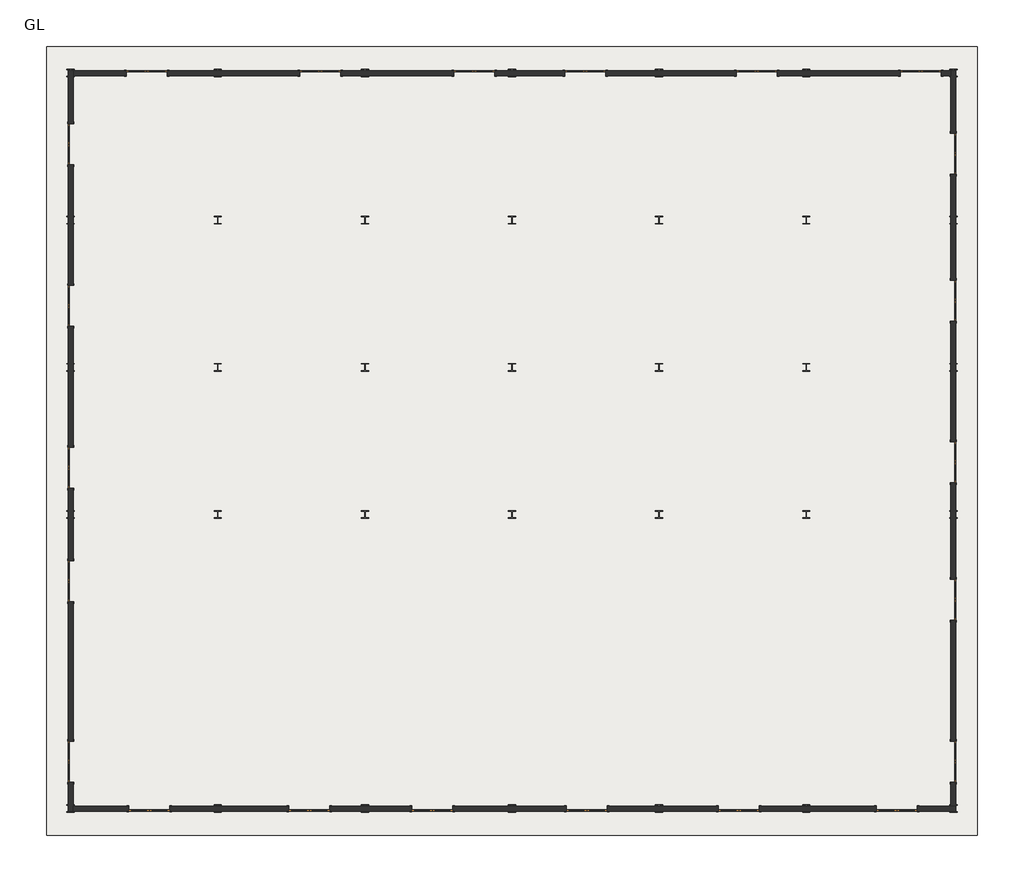
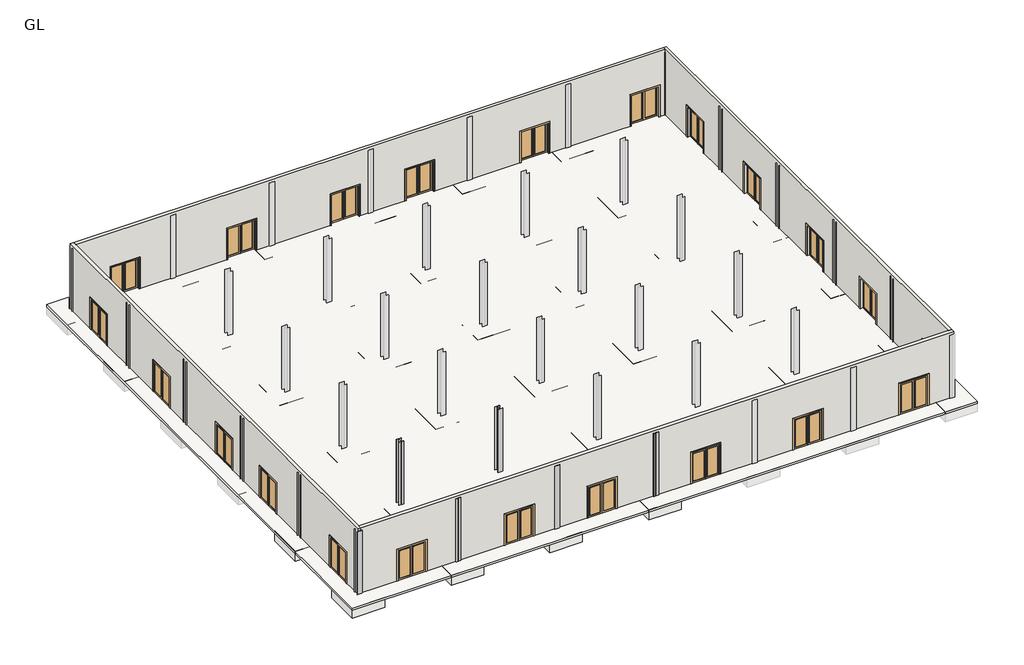
# One storey, part 1 of 2: 22 doors, 9 slabs, 7 columns, 4 walls.
"""IFC4 building model written with IfcOpenShell, lengths in millimetres."""

from ifc_helpers import new_model, si_unit, frame, origin, place, context, project, spatial, polyline, outline, extrude, faceted_brep, transform, mapped, element, save
from components import uc_universal_columns_column_uc305x305x97_28816581, m_door_double_glass_1700_x_2000mm_d5355b94, m_footing_rectangular_2200_x_2000_x_650mm_2_4a7b59ae

model = new_model("IFC4")

# Units and contexts
model_context = context("Model", 3, world=origin())
ifc_project = project(units=[si_unit("LENGTHUNIT", "METRE", prefix="MILLI")], contexts=[model_context])

# Site, building, storey
site = spatial("IfcSite", under=ifc_project)
building = spatial("IfcBuilding", under=site)
storey = spatial("IfcBuildingStorey", under=building, Name="GL", Elevation=-1812.3304639)

# Columns
placement = place(None, origin())
uc_universal_columns_column_uc305x305x97_shape = uc_universal_columns_column_uc305x305x97_28816581(model_context)
element("IfcColumn", 1, ObjectType="UC-Universal Columns-Column : UC305x305x97", at=placement, inside=storey, context=model_context, shape_type="MappedRepresentation", body=[
    mapped(uc_universal_columns_column_uc305x305x97_shape, transform((-18630.5493858, -6191.7308265, 0.0), x_axis=(1.0, 0.0, 0.0), y_axis=(0.0, 1.0, 0.0), z_axis=(0.0, 0.0, 1.0))),
])
element("IfcColumn", 2, ObjectType="UC-Universal Columns-Column : UC305x305x97", at=placement, inside=storey, context=model_context, shape_type="MappedRepresentation", body=[
    mapped(uc_universal_columns_column_uc305x305x97_shape, transform((-12534.5493858, -6191.7308265, 0.0), x_axis=(1.0, 0.0, 0.0), y_axis=(0.0, 1.0, 0.0), z_axis=(0.0, 0.0, 1.0))),
])
element("IfcColumn", 3, ObjectType="UC-Universal Columns-Column : UC305x305x97", at=placement, inside=storey, context=model_context, shape_type="MappedRepresentation", body=[
    mapped(uc_universal_columns_column_uc305x305x97_shape, transform((-6438.5493858, -6191.7308265, 0.0), x_axis=(1.0, 0.0, 0.0), y_axis=(0.0, 1.0, 0.0), z_axis=(0.0, 0.0, 1.0))),
])
element("IfcColumn", 4, ObjectType="UC-Universal Columns-Column : UC305x305x97", at=placement, inside=storey, context=model_context, shape_type="MappedRepresentation", body=[
    mapped(uc_universal_columns_column_uc305x305x97_shape, transform((-342.5493858, -6191.7308265, 0.0), x_axis=(1.0, 0.0, 0.0), y_axis=(0.0, 1.0, 0.0), z_axis=(0.0, 0.0, 1.0))),
])
element("IfcColumn", 5, ObjectType="UC-Universal Columns-Column : UC305x305x97", at=placement, inside=storey, context=model_context, shape_type="MappedRepresentation", body=[
    mapped(uc_universal_columns_column_uc305x305x97_shape, transform((-18630.5493858, -95.7308265, 0.0), x_axis=(1.0, 0.0, 0.0), y_axis=(0.0, 1.0, 0.0), z_axis=(0.0, 0.0, 1.0))),
])
element("IfcColumn", 6, ObjectType="UC-Universal Columns-Column : UC305x305x97", at=placement, inside=storey, context=model_context, shape_type="MappedRepresentation", body=[
    mapped(uc_universal_columns_column_uc305x305x97_shape, transform((-12534.5493858, -95.7308265, 0.0), x_axis=(1.0, 0.0, 0.0), y_axis=(0.0, 1.0, 0.0), z_axis=(0.0, 0.0, 1.0))),
])
element("IfcColumn", 7, ObjectType="UC-Universal Columns-Column : UC305x305x97", at=placement, inside=storey, context=model_context, shape_type="MappedRepresentation", body=[
    mapped(uc_universal_columns_column_uc305x305x97_shape, transform((-6438.5493858, -95.7308265, 0.0), x_axis=(1.0, 0.0, 0.0), y_axis=(0.0, 1.0, 0.0), z_axis=(0.0, 0.0, 1.0))),
])

# Doors
m_door_double_glass_1700_x_2000mm_shape = m_door_double_glass_1700_x_2000mm_d5355b94(model_context)
element("IfcDoor", 8, ObjectType="M_Door-Double-Glass : 1700 x 2000mm", at=placement, inside=storey, context=model_context, shape_type="MappedRepresentation", body=[
    mapped(m_door_double_glass_1700_x_2000mm_shape, transform((-3650.2445858, -6189.3495765, -1812.3304639), x_axis=(-1.0, 0.0, 0.0), y_axis=(0.0, -1.0, 0.0), z_axis=(0.0, 0.0, 1.0))),
])
element("IfcDoor", 9, ObjectType="M_Door-Double-Glass : 1700 x 2000mm", at=placement, inside=storey, context=model_context, shape_type="MappedRepresentation", body=[
    mapped(m_door_double_glass_1700_x_2000mm_shape, transform((2749.7554142, -6189.3495765, -1812.3304639), x_axis=(-1.0, 0.0, 0.0), y_axis=(0.0, -1.0, 0.0), z_axis=(0.0, 0.0, 1.0))),
])
element("IfcDoor", 10, ObjectType="M_Door-Double-Glass : 1700 x 2000mm", at=placement, inside=storey, context=model_context, shape_type="MappedRepresentation", body=[
    mapped(m_door_double_glass_1700_x_2000mm_shape, transform((-8292.3969858, 24285.5831235, -1812.3304639), x_axis=(1.0, 0.0, 0.0), y_axis=(0.0, 1.0, 0.0), z_axis=(0.0, 0.0, 1.0))),
])
element("IfcDoor", 11, ObjectType="M_Door-Double-Glass : 1700 x 2000mm", at=placement, inside=storey, context=model_context, shape_type="MappedRepresentation", body=[
    mapped(m_door_double_glass_1700_x_2000mm_shape, transform((9795.4506142, 24285.5831235, -1812.3304639), x_axis=(1.0, 0.0, 0.0), y_axis=(0.0, 1.0, 0.0), z_axis=(0.0, 0.0, 1.0))),
])
element("IfcDoor", 12, ObjectType="M_Door-Double-Glass : 1700 x 2000mm", at=placement, inside=storey, context=model_context, shape_type="MappedRepresentation", body=[
    mapped(m_door_double_glass_1700_x_2000mm_shape, transform((-15480.2445858, 24285.5831235, -1812.3304639), x_axis=(1.0, 0.0, 0.0), y_axis=(0.0, 1.0, 0.0), z_axis=(0.0, 0.0, 1.0))),
])
element("IfcDoor", 13, ObjectType="M_Door-Double-Glass : 1700 x 2000mm", at=placement, inside=storey, context=model_context, shape_type="MappedRepresentation", body=[
    mapped(m_door_double_glass_1700_x_2000mm_shape, transform((-1904.5493858, 24285.5831235, -1812.3304639), x_axis=(1.0, 0.0, 0.0), y_axis=(0.0, 1.0, 0.0), z_axis=(0.0, 0.0, 1.0))),
])
element("IfcDoor", 14, ObjectType="M_Door-Double-Glass : 1700 x 2000mm", at=placement, inside=storey, context=model_context, shape_type="MappedRepresentation", body=[
    mapped(m_door_double_glass_1700_x_2000mm_shape, transform((16595.4506142, 24285.5831235, -1812.3304639), x_axis=(1.0, 0.0, 0.0), y_axis=(0.0, 1.0, 0.0), z_axis=(0.0, 0.0, 1.0))),
])
element("IfcDoor", 15, ObjectType="M_Door-Double-Glass : 1700 x 2000mm", at=placement, inside=storey, context=model_context, shape_type="MappedRepresentation", body=[
    mapped(m_door_double_glass_1700_x_2000mm_shape, transform((2695.4506142, 24285.5831235, -1812.3304639), x_axis=(1.0, 0.0, 0.0), y_axis=(0.0, 1.0, 0.0), z_axis=(0.0, 0.0, 1.0))),
])
element("IfcDoor", 16, ObjectType="M_Door-Double-Glass : 1700 x 2000mm", at=placement, inside=storey, context=model_context, shape_type="MappedRepresentation", body=[
    mapped(m_door_double_glass_1700_x_2000mm_shape, transform((-18627.8633358, 21337.9643735, -1812.3304639), x_axis=(0.0, 1.0, 0.0), y_axis=(-1.0, 0.0, 0.0), z_axis=(0.0, 0.0, 1.0))),
])
element("IfcDoor", 17, ObjectType="M_Door-Double-Glass : 1700 x 2000mm", at=placement, inside=storey, context=model_context, shape_type="MappedRepresentation", body=[
    mapped(m_door_double_glass_1700_x_2000mm_shape, transform((-18627.8633358, 14637.9643735, -1812.3304639), x_axis=(0.0, 1.0, 0.0), y_axis=(-1.0, 0.0, 0.0), z_axis=(0.0, 0.0, 1.0))),
])
element("IfcDoor", 18, ObjectType="M_Door-Double-Glass : 1700 x 2000mm", at=placement, inside=storey, context=model_context, shape_type="MappedRepresentation", body=[
    mapped(m_door_double_glass_1700_x_2000mm_shape, transform((-18627.8633358, 7937.9643735, -1812.3304639), x_axis=(0.0, 1.0, 0.0), y_axis=(-1.0, 0.0, 0.0), z_axis=(0.0, 0.0, 1.0))),
])
element("IfcDoor", 19, ObjectType="M_Door-Double-Glass : 1700 x 2000mm", at=placement, inside=storey, context=model_context, shape_type="MappedRepresentation", body=[
    mapped(m_door_double_glass_1700_x_2000mm_shape, transform((-18627.8633358, 3237.9643735, -1812.3304639), x_axis=(0.0, 1.0, 0.0), y_axis=(-1.0, 0.0, 0.0), z_axis=(0.0, 0.0, 1.0))),
])
element("IfcDoor", 20, ObjectType="M_Door-Double-Glass : 1700 x 2000mm", at=placement, inside=storey, context=model_context, shape_type="MappedRepresentation", body=[
    mapped(m_door_double_glass_1700_x_2000mm_shape, transform((-18627.8633358, -4241.7308265, -1812.3304639), x_axis=(0.0, 1.0, 0.0), y_axis=(-1.0, 0.0, 0.0), z_axis=(0.0, 0.0, 1.0))),
])
element("IfcDoor", 21, ObjectType="M_Door-Double-Glass : 1700 x 2000mm", at=placement, inside=storey, context=model_context, shape_type="MappedRepresentation", body=[
    mapped(m_door_double_glass_1700_x_2000mm_shape, transform((17943.0693642, -4241.7308265, -1812.3304639), x_axis=(0.0, -1.0, 0.0), y_axis=(1.0, 0.0, 0.0), z_axis=(0.0, 0.0, 1.0))),
])
element("IfcDoor", 22, ObjectType="M_Door-Double-Glass : 1700 x 2000mm", at=placement, inside=storey, context=model_context, shape_type="MappedRepresentation", body=[
    mapped(m_door_double_glass_1700_x_2000mm_shape, transform((17943.0693642, 2458.2691735, -1812.3304639), x_axis=(0.0, -1.0, 0.0), y_axis=(1.0, 0.0, 0.0), z_axis=(0.0, 0.0, 1.0))),
])
element("IfcDoor", 23, ObjectType="M_Door-Double-Glass : 1700 x 2000mm", at=placement, inside=storey, context=model_context, shape_type="MappedRepresentation", body=[
    mapped(m_door_double_glass_1700_x_2000mm_shape, transform((17943.0693642, 8158.2691735, -1812.3304639), x_axis=(0.0, -1.0, 0.0), y_axis=(1.0, 0.0, 0.0), z_axis=(0.0, 0.0, 1.0))),
])
element("IfcDoor", 24, ObjectType="M_Door-Double-Glass : 1700 x 2000mm", at=placement, inside=storey, context=model_context, shape_type="MappedRepresentation", body=[
    mapped(m_door_double_glass_1700_x_2000mm_shape, transform((17943.0693642, 14858.2691735, -1812.3304639), x_axis=(0.0, -1.0, 0.0), y_axis=(1.0, 0.0, 0.0), z_axis=(0.0, 0.0, 1.0))),
])
element("IfcDoor", 25, ObjectType="M_Door-Double-Glass : 1700 x 2000mm", at=placement, inside=storey, context=model_context, shape_type="MappedRepresentation", body=[
    mapped(m_door_double_glass_1700_x_2000mm_shape, transform((-15380.2445858, -6189.3495765, -1812.3304639), x_axis=(-1.0, 0.0, 0.0), y_axis=(0.0, -1.0, 0.0), z_axis=(0.0, 0.0, 1.0))),
])
element("IfcDoor", 26, ObjectType="M_Door-Double-Glass : 1700 x 2000mm", at=placement, inside=storey, context=model_context, shape_type="MappedRepresentation", body=[
    mapped(m_door_double_glass_1700_x_2000mm_shape, transform((-8750.2445858, -6189.3495765, -1812.3304639), x_axis=(-1.0, 0.0, 0.0), y_axis=(0.0, -1.0, 0.0), z_axis=(0.0, 0.0, 1.0))),
])
element("IfcDoor", 27, ObjectType="M_Door-Double-Glass : 1700 x 2000mm", at=placement, inside=storey, context=model_context, shape_type="MappedRepresentation", body=[
    mapped(m_door_double_glass_1700_x_2000mm_shape, transform((9049.7554142, -6189.3495765, -1812.3304639), x_axis=(-1.0, 0.0, 0.0), y_axis=(0.0, -1.0, 0.0), z_axis=(0.0, 0.0, 1.0))),
])
element("IfcDoor", 28, ObjectType="M_Door-Double-Glass : 1700 x 2000mm", at=placement, inside=storey, context=model_context, shape_type="MappedRepresentation", body=[
    mapped(m_door_double_glass_1700_x_2000mm_shape, transform((15595.4506142, -6189.3495765, -1812.3304639), x_axis=(-1.0, 0.0, 0.0), y_axis=(0.0, -1.0, 0.0), z_axis=(0.0, 0.0, 1.0))),
])
element("IfcDoor", 29, ObjectType="M_Door-Double-Glass : 1700 x 2000mm", at=placement, inside=storey, context=model_context, shape_type="MappedRepresentation", body=[
    mapped(m_door_double_glass_1700_x_2000mm_shape, transform((17943.0693642, 20937.9643735, -1812.3304639), x_axis=(0.0, -1.0, 0.0), y_axis=(1.0, 0.0, 0.0), z_axis=(0.0, 0.0, 1.0))),
])

# Slabs
element("IfcSlab", 30, ObjectType="Generic 150mm", at=placement, inside=storey, context=model_context, shape_type="SweptSolid", body=[
    extrude(outline(polyline([(18945.4506142, 25388.2691735), (18945.4506142, -7291.7308265), (-19630.5493858, -7291.7308265), (-19630.5493858, 25388.2691735), (18945.4506142, 25388.2691735)])), frame((0.0, 0.0, -1962.3304639), z_axis=(0.0, 0.0, 1.0), x_axis=(1.0, 0.0, 0.0)), (0.0, 0.0, 1.0), 150.0),
])
m_footing_rectangular_2200_x_2000_x_650mm_2_shape = m_footing_rectangular_2200_x_2000_x_650mm_2_4a7b59ae(model_context)
element("IfcSlab", 31, ObjectType="M_Footing-Rectangular : 2200 x 2000 x 650mm 2", at=placement, inside=storey, context=model_context, shape_type="MappedRepresentation", body=[
    mapped(m_footing_rectangular_2200_x_2000_x_650mm_2_shape, transform((-18630.5493858, -6191.7308265, -1812.3304639), x_axis=(1.0, 0.0, 0.0), y_axis=(0.0, 1.0, 0.0), z_axis=(0.0, 0.0, 1.0))),
])
element("IfcSlab", 32, ObjectType="M_Footing-Rectangular : 2200 x 2000 x 650mm 2", at=placement, inside=storey, context=model_context, shape_type="MappedRepresentation", body=[
    mapped(m_footing_rectangular_2200_x_2000_x_650mm_2_shape, transform((-12534.5493858, -6191.7308265, -1812.3304639), x_axis=(1.0, 0.0, 0.0), y_axis=(0.0, 1.0, 0.0), z_axis=(0.0, 0.0, 1.0))),
])
element("IfcSlab", 33, ObjectType="M_Footing-Rectangular : 2200 x 2000 x 650mm 2", at=placement, inside=storey, context=model_context, shape_type="MappedRepresentation", body=[
    mapped(m_footing_rectangular_2200_x_2000_x_650mm_2_shape, transform((-6438.5493858, -6191.7308265, -1812.3304639), x_axis=(1.0, 0.0, 0.0), y_axis=(0.0, 1.0, 0.0), z_axis=(0.0, 0.0, 1.0))),
])
element("IfcSlab", 34, ObjectType="M_Footing-Rectangular : 2200 x 2000 x 650mm 2", at=placement, inside=storey, context=model_context, shape_type="MappedRepresentation", body=[
    mapped(m_footing_rectangular_2200_x_2000_x_650mm_2_shape, transform((-342.5493858, -6191.7308265, -1812.3304639), x_axis=(1.0, 0.0, 0.0), y_axis=(0.0, 1.0, 0.0), z_axis=(0.0, 0.0, 1.0))),
])
element("IfcSlab", 35, ObjectType="M_Footing-Rectangular : 2200 x 2000 x 650mm 2", at=placement, inside=storey, context=model_context, shape_type="MappedRepresentation", body=[
    mapped(m_footing_rectangular_2200_x_2000_x_650mm_2_shape, transform((-18630.5493858, -95.7308265, -1812.3304639), x_axis=(1.0, 0.0, 0.0), y_axis=(0.0, 1.0, 0.0), z_axis=(0.0, 0.0, 1.0))),
])
element("IfcSlab", 36, ObjectType="M_Footing-Rectangular : 2200 x 2000 x 650mm 2", at=placement, inside=storey, context=model_context, shape_type="MappedRepresentation", body=[
    mapped(m_footing_rectangular_2200_x_2000_x_650mm_2_shape, transform((-12534.5493858, -95.7308265, -1812.3304639), x_axis=(1.0, 0.0, 0.0), y_axis=(0.0, 1.0, 0.0), z_axis=(0.0, 0.0, 1.0))),
])
element("IfcSlab", 37, ObjectType="M_Footing-Rectangular : 2200 x 2000 x 650mm 2", at=placement, inside=storey, context=model_context, shape_type="MappedRepresentation", body=[
    mapped(m_footing_rectangular_2200_x_2000_x_650mm_2_shape, transform((-6438.5493858, -95.7308265, -1812.3304639), x_axis=(1.0, 0.0, 0.0), y_axis=(0.0, 1.0, 0.0), z_axis=(0.0, 0.0, 1.0))),
])
element("IfcSlab", 38, ObjectType="M_Footing-Rectangular : 2200 x 2000 x 650mm 2", at=placement, inside=storey, context=model_context, shape_type="MappedRepresentation", body=[
    mapped(m_footing_rectangular_2200_x_2000_x_650mm_2_shape, transform((-342.5493858, -95.7308265, -1812.3304639), x_axis=(1.0, 0.0, 0.0), y_axis=(0.0, 1.0, 0.0), z_axis=(0.0, 0.0, 1.0))),
])

# Walls
element("IfcWall", 39, ObjectType="Generic - 200mm", at=placement, inside=storey, context=model_context, shape_type="Brep", body=[
    faceted_brep([(-18730.2445858, 2387.9643735, -1812.3304639), (-18730.2445858, -3391.7308265, -1812.3304639), (-18730.2445858, -3391.7308265, 187.6695361), (-18730.2445858, -5091.7308265, 187.6695361), (-18730.2445858, -5091.7308265, -1812.3304639), (-18730.2445858, -6291.7308265, -1812.3304639), (-18730.2445858, -6291.7308265, 2454.6695361), (-18730.2445858, 24387.9643735, 2454.6695361), (-18730.2445858, 24387.9643735, -1812.3304639), (-18730.2445858, 22187.9643735, -1812.3304639), (-18730.2445858, 22187.9643735, 187.6695361), (-18730.2445858, 20487.9643735, 187.6695361), (-18730.2445858, 20487.9643735, -1812.3304639), (-18730.2445858, 15487.9643735, -1812.3304639), (-18730.2445858, 15487.9643735, 187.6695361), (-18730.2445858, 13787.9643735, 187.6695361), (-18730.2445858, 13787.9643735, -1812.3304639), (-18730.2445858, 8787.9643735, -1812.3304639), (-18730.2445858, 8787.9643735, 187.6695361), (-18730.2445858, 7087.9643735, 187.6695361), (-18730.2445858, 7087.9643735, -1812.3304639), (-18730.2445858, 4087.9643735, -1812.3304639), (-18730.2445858, 4087.9643735, 187.6695361), (-18730.2445858, 2387.9643735, 187.6695361), (-18530.2445858, -3391.7308265, 187.6695361), (-18530.2445858, -3391.7308265, -1812.3304639), (-18530.2445858, 2387.9643735, -1812.3304639), (-18530.2445858, 2387.9643735, 187.6695361), (-18530.2445858, 4087.9643735, 187.6695361), (-18530.2445858, 4087.9643735, -1812.3304639), (-18530.2445858, 7087.9643735, -1812.3304639), (-18530.2445858, 7087.9643735, 187.6695361), (-18530.2445858, 8787.9643735, 187.6695361), (-18530.2445858, 8787.9643735, -1812.3304639), (-18530.2445858, 13787.9643735, -1812.3304639), (-18530.2445858, 13787.9643735, 187.6695361), (-18530.2445858, 15487.9643735, 187.6695361), (-18530.2445858, 15487.9643735, -1812.3304639), (-18530.2445858, 20487.9643735, -1812.3304639), (-18530.2445858, 20487.9643735, 187.6695361), (-18530.2445858, 22187.9643735, 187.6695361), (-18530.2445858, 22187.9643735, -1812.3304639), (-18530.2445858, 24187.9643735, -1812.3304639), (-18530.2445858, 24387.9643735, -1812.3304639), (-18530.2445858, 24387.9643735, 2454.6695361), (-18530.2445858, 24187.9643735, 2454.6695361), (-18530.2445858, -6091.7308265, 2454.6695361), (-18530.2445858, -6291.7308265, 2454.6695361), (-18530.2445858, -6291.7308265, -1812.3304639), (-18530.2445858, -6091.7308265, -1812.3304639), (-18530.2445858, -5091.7308265, -1812.3304639), (-18530.2445858, -5091.7308265, 187.6695361)], [[[0, 1, 2, 3, 4, 5, 6, 7, 8, 9, 10, 11, 12, 13, 14, 15, 16, 17, 18, 19, 20, 21, 22, 23]], [[24, 25, 26, 27, 28, 29, 30, 31, 32, 33, 34, 35, 36, 37, 38, 39, 40, 41, 42, 43, 44, 45, 46, 47, 48, 49, 50, 51]], [[43, 42, 41, 9, 8]], [[38, 37, 13, 12]], [[34, 33, 17, 16]], [[30, 29, 21, 20]], [[26, 25, 1, 0]], [[50, 49, 48, 5, 4]], [[7, 6, 47, 46, 45, 44]], [[6, 5, 48, 47]], [[8, 7, 44, 43]], [[10, 9, 41, 40]], [[11, 10, 40, 39]], [[12, 11, 39, 38]], [[14, 13, 37, 36]], [[15, 14, 36, 35]], [[16, 15, 35, 34]], [[18, 17, 33, 32]], [[19, 18, 32, 31]], [[20, 19, 31, 30]], [[22, 21, 29, 28]], [[23, 22, 28, 27]], [[0, 23, 27, 26]], [[2, 1, 25, 24]], [[3, 2, 24, 51]], [[4, 3, 51, 50]]]),
])
element("IfcWall", 40, ObjectType="Generic - 200mm", at=placement, inside=storey, context=model_context, shape_type="Brep", body=[
    faceted_brep([(9899.7554142, -6291.7308265, -1812.3304639), (14745.4506142, -6291.7308265, -1812.3304639), (14745.4506142, -6291.7308265, 187.6695361), (16445.4506142, -6291.7308265, 187.6695361), (16445.4506142, -6291.7308265, -1812.3304639), (18045.4506142, -6291.7308265, -1812.3304639), (18045.4506142, -6291.7308265, 2454.6695361), (-18530.2445858, -6291.7308265, 2454.6695361), (-18530.2445858, -6291.7308265, -1812.3304639), (-16230.2445858, -6291.7308265, -1812.3304639), (-16230.2445858, -6291.7308265, 187.6695361), (-14530.2445858, -6291.7308265, 187.6695361), (-14530.2445858, -6291.7308265, -1812.3304639), (-9600.2445858, -6291.7308265, -1812.3304639), (-9600.2445858, -6291.7308265, 187.6695361), (-7900.2445858, -6291.7308265, 187.6695361), (-7900.2445858, -6291.7308265, -1812.3304639), (-4500.2445858, -6291.7308265, -1812.3304639), (-4500.2445858, -6291.7308265, 187.6695361), (-2800.2445858, -6291.7308265, 187.6695361), (-2800.2445858, -6291.7308265, -1812.3304639), (1899.7554142, -6291.7308265, -1812.3304639), (1899.7554142, -6291.7308265, 187.6695361), (3599.7554142, -6291.7308265, 187.6695361), (3599.7554142, -6291.7308265, -1812.3304639), (8199.7554142, -6291.7308265, -1812.3304639), (8199.7554142, -6291.7308265, 187.6695361), (9899.7554142, -6291.7308265, 187.6695361), (14745.4506142, -6091.7308265, 187.6695361), (14745.4506142, -6091.7308265, -1812.3304639), (9899.7554142, -6091.7308265, -1812.3304639), (9899.7554142, -6091.7308265, 187.6695361), (8199.7554142, -6091.7308265, 187.6695361), (8199.7554142, -6091.7308265, -1812.3304639), (3599.7554142, -6091.7308265, -1812.3304639), (3599.7554142, -6091.7308265, 187.6695361), (1899.7554142, -6091.7308265, 187.6695361), (1899.7554142, -6091.7308265, -1812.3304639), (-2800.2445858, -6091.7308265, -1812.3304639), (-2800.2445858, -6091.7308265, 187.6695361), (-4500.2445858, -6091.7308265, 187.6695361), (-4500.2445858, -6091.7308265, -1812.3304639), (-7900.2445858, -6091.7308265, -1812.3304639), (-7900.2445858, -6091.7308265, 187.6695361), (-9600.2445858, -6091.7308265, 187.6695361), (-9600.2445858, -6091.7308265, -1812.3304639), (-14530.2445858, -6091.7308265, -1812.3304639), (-14530.2445858, -6091.7308265, 187.6695361), (-16230.2445858, -6091.7308265, 187.6695361), (-16230.2445858, -6091.7308265, -1812.3304639), (-18530.2445858, -6091.7308265, -1812.3304639), (-18530.2445858, -6091.7308265, 2454.6695361), (17845.4506142, -6091.7308265, 2454.6695361), (18045.4506142, -6091.7308265, 2454.6695361), (18045.4506142, -6091.7308265, -1812.3304639), (17845.4506142, -6091.7308265, -1812.3304639), (16445.4506142, -6091.7308265, -1812.3304639), (16445.4506142, -6091.7308265, 187.6695361)], [[[0, 1, 2, 3, 4, 5, 6, 7, 8, 9, 10, 11, 12, 13, 14, 15, 16, 17, 18, 19, 20, 21, 22, 23, 24, 25, 26, 27]], [[28, 29, 30, 31, 32, 33, 34, 35, 36, 37, 38, 39, 40, 41, 42, 43, 44, 45, 46, 47, 48, 49, 50, 51, 52, 53, 54, 55, 56, 57]], [[38, 37, 21, 20]], [[50, 49, 9, 8]], [[42, 41, 17, 16]], [[46, 45, 13, 12]], [[34, 33, 25, 24]], [[30, 29, 1, 0]], [[56, 55, 54, 5, 4]], [[7, 6, 53, 52, 51]], [[8, 7, 51, 50]], [[6, 5, 54, 53]], [[18, 17, 41, 40]], [[19, 18, 40, 39]], [[20, 19, 39, 38]], [[22, 21, 37, 36]], [[23, 22, 36, 35]], [[24, 23, 35, 34]], [[10, 9, 49, 48]], [[11, 10, 48, 47]], [[12, 11, 47, 46]], [[14, 13, 45, 44]], [[15, 14, 44, 43]], [[16, 15, 43, 42]], [[26, 25, 33, 32]], [[27, 26, 32, 31]], [[0, 27, 31, 30]], [[2, 1, 29, 28]], [[3, 2, 28, 57]], [[4, 3, 57, 56]]]),
])
element("IfcWall", 41, ObjectType="Generic - 200mm", at=placement, inside=storey, context=model_context, shape_type="Brep", body=[
    faceted_brep([(18045.4506142, 15708.2691735, -1812.3304639), (18045.4506142, 20087.9643735, -1812.3304639), (18045.4506142, 20087.9643735, 187.6695361), (18045.4506142, 21787.9643735, 187.6695361), (18045.4506142, 21787.9643735, -1812.3304639), (18045.4506142, 24387.9643735, -1812.3304639), (18045.4506142, 24387.9643735, 2454.6695361), (18045.4506142, -6091.7308265, 2454.6695361), (18045.4506142, -6091.7308265, -1812.3304639), (18045.4506142, -5091.7308265, -1812.3304639), (18045.4506142, -5091.7308265, 187.6695361), (18045.4506142, -3391.7308265, 187.6695361), (18045.4506142, -3391.7308265, -1812.3304639), (18045.4506142, 1608.2691735, -1812.3304639), (18045.4506142, 1608.2691735, 187.6695361), (18045.4506142, 3308.2691735, 187.6695361), (18045.4506142, 3308.2691735, -1812.3304639), (18045.4506142, 7308.2691735, -1812.3304639), (18045.4506142, 7308.2691735, 187.6695361), (18045.4506142, 9008.2691735, 187.6695361), (18045.4506142, 9008.2691735, -1812.3304639), (18045.4506142, 14008.2691735, -1812.3304639), (18045.4506142, 14008.2691735, 187.6695361), (18045.4506142, 15708.2691735, 187.6695361), (17845.4506142, 20087.9643735, 187.6695361), (17845.4506142, 20087.9643735, -1812.3304639), (17845.4506142, 15708.2691735, -1812.3304639), (17845.4506142, 15708.2691735, 187.6695361), (17845.4506142, 14008.2691735, 187.6695361), (17845.4506142, 14008.2691735, -1812.3304639), (17845.4506142, 9008.2691735, -1812.3304639), (17845.4506142, 9008.2691735, 187.6695361), (17845.4506142, 7308.2691735, 187.6695361), (17845.4506142, 7308.2691735, -1812.3304639), (17845.4506142, 3308.2691735, -1812.3304639), (17845.4506142, 3308.2691735, 187.6695361), (17845.4506142, 1608.2691735, 187.6695361), (17845.4506142, 1608.2691735, -1812.3304639), (17845.4506142, -3391.7308265, -1812.3304639), (17845.4506142, -3391.7308265, 187.6695361), (17845.4506142, -5091.7308265, 187.6695361), (17845.4506142, -5091.7308265, -1812.3304639), (17845.4506142, -6091.7308265, -1812.3304639), (17845.4506142, -6091.7308265, 2454.6695361), (17845.4506142, 24187.9643735, 2454.6695361), (17845.4506142, 24387.9643735, 2454.6695361), (17845.4506142, 24387.9643735, -1812.3304639), (17845.4506142, 24187.9643735, -1812.3304639), (17845.4506142, 21787.9643735, -1812.3304639), (17845.4506142, 21787.9643735, 187.6695361)], [[[0, 1, 2, 3, 4, 5, 6, 7, 8, 9, 10, 11, 12, 13, 14, 15, 16, 17, 18, 19, 20, 21, 22, 23]], [[24, 25, 26, 27, 28, 29, 30, 31, 32, 33, 34, 35, 36, 37, 38, 39, 40, 41, 42, 43, 44, 45, 46, 47, 48, 49]], [[42, 41, 9, 8]], [[38, 37, 13, 12]], [[34, 33, 17, 16]], [[30, 29, 21, 20]], [[26, 25, 1, 0]], [[48, 47, 46, 5, 4]], [[7, 6, 45, 44, 43]], [[8, 7, 43, 42]], [[6, 5, 46, 45]], [[10, 9, 41, 40]], [[11, 10, 40, 39]], [[12, 11, 39, 38]], [[14, 13, 37, 36]], [[15, 14, 36, 35]], [[16, 15, 35, 34]], [[18, 17, 33, 32]], [[19, 18, 32, 31]], [[20, 19, 31, 30]], [[22, 21, 29, 28]], [[23, 22, 28, 27]], [[0, 23, 27, 26]], [[2, 1, 25, 24]], [[3, 2, 24, 49]], [[4, 3, 49, 48]]]),
])
element("IfcWall", 42, ObjectType="Generic - 200mm", at=placement, inside=storey, context=model_context, shape_type="SweptSolid", body=[
    extrude(outline(polyline([(187.6695361, 3545.4506142), (-1812.3304639, 3545.4506142), (-1812.3304639, 8945.4506142), (187.6695361, 8945.4506142), (187.6695361, 10645.4506142), (-1812.3304639, 10645.4506142), (-1812.3304639, 15745.4506142), (187.6695361, 15745.4506142), (187.6695361, 17445.4506142), (-1812.3304639, 17445.4506142), (-1812.3304639, 17845.4506142), (2454.6695361, 17845.4506142), (2454.6695361, -18530.2445858), (-1812.3304639, -18530.2445858), (-1812.3304639, -16330.2445858), (187.6695361, -16330.2445858), (187.6695361, -14630.2445858), (-1812.3304639, -14630.2445858), (-1812.3304639, -9142.3969858), (187.6695361, -9142.3969858), (187.6695361, -7442.3969858), (-1812.3304639, -7442.3969858), (-1812.3304639, -2754.5493858), (187.6695361, -2754.5493858), (187.6695361, -1054.5493858), (-1812.3304639, -1054.5493858), (-1812.3304639, 1845.4506142), (187.6695361, 1845.4506142), (187.6695361, 3545.4506142)])), frame((0.0, 24187.9643735, 0.0), z_axis=(0.0, 1.0, 0.0), x_axis=(0.0, 0.0, 1.0)), (0.0, 0.0, 1.0), 200.0),
])

save(model, "model.ifc")

# Revit data of these elements
# Grids (mm)
#   "1": line (20610.061, -6191.731) -> (-20257.131, -6191.731)
#   "2": line (20610.061, -95.731) -> (-20257.131, -95.731)
#   "3": line (20610.061, 6000.269) -> (-20257.131, 6000.269)
#   "4": line (20610.061, 12096.269) -> (-20257.131, 12096.269)
#   "5": line (20610.061, 18192.269) -> (-20257.131, 18192.269)
#   "6": line (20610.061, 24288.269) -> (-20257.131, 24288.269)
#   "8": line (-12534.549, 28626.482) -> (-12534.549, -10472.495)
#   "9": line (-6438.549, 28626.482) -> (-6438.549, -10472.495)
#   "10": line (-342.549, 28626.482) -> (-342.549, -10472.495)
#   "11": line (5753.451, 28626.482) -> (5753.451, -10472.495)
#   "12": line (11849.451, 28626.482) -> (11849.451, -10472.495)
#   "13": line (17945.451, 28626.482) -> (17945.451, -10472.495)
#   "7": line (-18630.549, 28626.482) -> (-18630.549, -10472.495)
# Type "UC-Universal Columns-Column : UC305x305x97"
#   Section Name Key = "UC305x305x97"
#   Width = 30.53 cm
#   Web Thickness = 0.99 cm
#   Web Fillet = 1.52 cm
#   Warping Constant = 1560000.0 cm⁶
#   Torsional Moment of Inertia = 91.20 cm⁴
#   Section Area = 123.0 cm²
#   Plastic Modulus weak axis = 726.0 cm³
#   Plastic Modulus strong axis = 1592.0 cm³
#   Nominal Weight = 96.8996 kgf/m
#   Moment of Inertia weak axis = 7308.00 cm⁴
#   Moment of Inertia strong axis = 22249.00 cm⁴
#   Height = 30.79 cm
#   Flange Thickness = 1.54 cm
#   Elastic Modulus weak axis = 479.0 cm³
#   Elastic Modulus strong axis = 1445.0 cm³
#   Centroid Vertical = 15.395 cm
#   Centroid Horizontal = 15.265 cm
#   Bolt Spacing = 14.0 cm
#   Structural Material [instance default] = Metal - Steel 43-275
#   Type Comments = ""
#   Assembly Code = ""
# Type "M_Door-Double-Glass : 1700 x 2000mm"
#   Type Mark = "40"
#   Construction Type Id = "opn-d45"
#   Assembly Code = "C1020"
#   Analytic Construction = "Wood frame, double glass door "
#   W = 850 mm
#   Thickness = 50 mm
#   Thermal Resistance (R) = 0.31964 (m²·K)/W
#   Swing Angle [instance default] = 90.00°
#   Heat Transfer Coefficient (U) = 3.12872 W/(m²·K)
#   Height = 2000 mm
#   Bottom Rail = 100 mm
#   Top Rail = 100 mm
#   Stiles = 100 mm
#   Trim Projection = 25 mm
#   Trim Width = 80 mm
#   Width = 1700 mm
#   Define Thermal Properties by = 1
#   Glazing = Glass
#   Panel Material = Wood - Birch - Solid Stained Light Low Gloss
#   Trim Material = Paint - Sienna
#   Visual Light Transmittance = 0
#   Solar Heat Gain Coefficient = 0
#   Function = (empty or 0)
#   Wall Closure = (empty or 0)
# Type "Generic 150mm"
#   Function = 0
#   Layers, outside or top first: 150 mm "Render, Tan, Textured" (function 1)
# Type "M_Footing-Rectangular : 2200 x 2000 x 650mm 2"
#   Width = 2000 mm
#   Length = 2200 mm
#   Foundation Thickness = 650 mm
#   Structural Material [instance default] = Concrete, Cast-in-Place gray
#   Assembly Code = ""
# Type "Generic - 200mm"
#   Layers, outside or top first: 200 mm "Door - Frame" (function 1)
# Elements 1, 2, 3, 4, 5, 6, 7 (IfcColumn, "UC-Universal Columns-Column : UC305x305x97")
#   Structural Material = Metal - Steel 43-275
#   Phase Created = New Construction
#   Materials on its faces: "Metal - Steel 43-275"
# Elements 8, 9, 10, 11, 12, 13, 14, 15, 16, 17, 18, 19, 20, 21, 22, 23, 24, 25, 26, 27, 28, 29 (IfcDoor, "M_Door-Double-Glass : 1700 x 2000mm")
#   Swing Angle = 90.00°
#   Phase Created = New Construction
#   Materials on its faces: "Wood - Birch - Solid Stained Light Low Gloss", "Paint - Sienna", "Glass"
# Element 30 (IfcSlab, "Generic 150mm")
#   Height Offset From Level = 0 mm
#   Phase Created = New Construction
#   Materials on its faces: "Render, Tan, Textured"
# Elements 31, 32, 33, 34, 35, 36, 37, 38 (IfcSlab, "M_Footing-Rectangular : 2200 x 2000 x 650mm 2")
#   Structural Material = Concrete, Cast-in-Place gray
#   Phase Created = New Construction
#   Materials on its faces: "Concrete, Cast-in-Place gray"
# Elements 39, 40, 41, 42 (IfcWall, "Generic - 200mm")
#   Top Offset = 0 mm
#   Base Offset = 0 mm
#   wall height = 4267 mm
#   Phase Created = New Construction
#   Base Constraint = GL
#   Top Constraint = FIRST FLOOR
#   Materials on its faces: "Door - Frame"
# Materials
#   "Metal - Steel 43-275": class "Metal", colour RGB 247 247 247, transparency 0, Cost = 0
#   "Glass": class "Glass", colour RGB 0 128 192, transparency 0.9, Description = "Soda Lime Glass", Cost = 0
#   "Wood - Birch - Solid Stained Light Low Gloss": class "Wood", colour RGB 210 159 95, transparency 0, Cost = 0
#   "Paint - Sienna": colour RGB 118 70 51, transparency 0, Cost = 0
#   "Render, Tan, Textured": class "Generic", colour RGB 196 158 130, transparency 0, Description = "physical material", Cost = 0
#   "Concrete, Cast-in-Place gray": class "Concrete", colour RGB 192 192 192, transparency 0, Description = "Cast-in-place concrete", Cost = 0
#   "Door - Frame": colour RGB 118 70 51, transparency 0, Cost = 0
